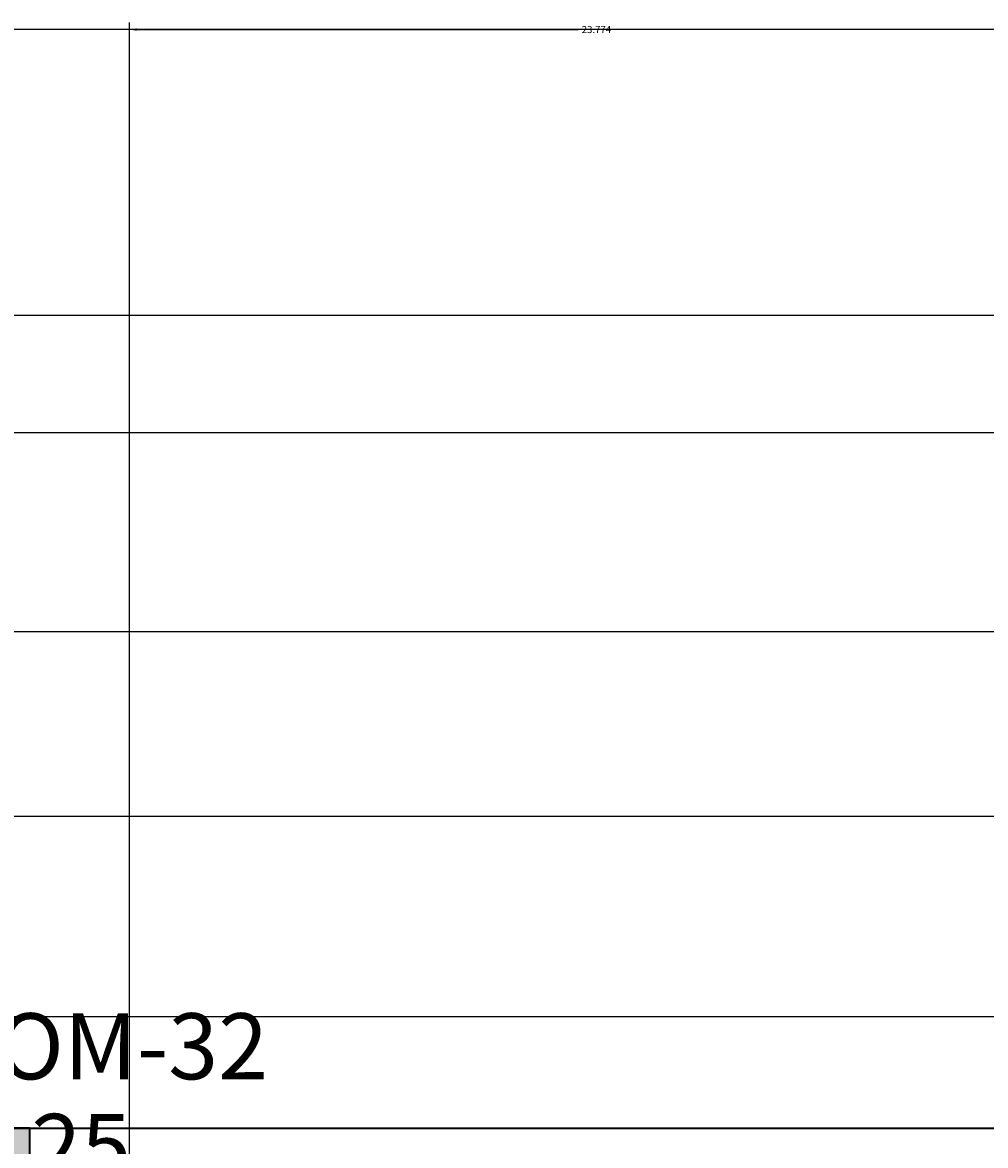
# Model space of a CAD drawing. Units: inches. Extents: x 23 to 132, y 5 to 105.
# Tile 13 of 14: x 81 to 105, y 77 to 105. Entities that reach past the tile are written whole.
import ezdxf

# ---------------------------------------------------------------- set-up
doc = ezdxf.new("R2010")
doc.units = ezdxf.units.IN
doc.header["$MEASUREMENT"] = 0
for name, color, linetype, lineweight in [('A-ANNO-DIMS', 2, 'Continuous', 18), ('E-ANNO-IDEN', 4, 'Continuous', 18), ('E-ANNO-TEXT', 3, 'Continuous', 18), ('E-SYMB', 1, 'Continuous', 35), ('E-SYMB-PATT', 1, 'Continuous', 18)]:
    doc.layers.add(name, color=color, linetype=linetype, lineweight=lineweight)
doc.styles.get("Standard").update_dxf_attribs({"font": 'arial.ttf'})
doc.dimstyles.get("Standard").update_dxf_attribs({"dimtxt": 0.18, "dimasz": 0.18, "dimexe": 0.18, "dimexo": 0.0625, "dimgap": 0.09, "dimtad": 0, "dimtih": 1, "dimtoh": 1, "dimdec": 4, "dimzin": 0, "dimdsep": 46, "dimtxsty": 'Standard', "dimcen": 0.09, "dimadec": 0, "dimazin": 0, "dimtfac": 1, "dimtdec": 4, "dimtofl": 0, "dimtmove": 0, "dimatfit": 3, "dimfxl": 1, "dimtolj": 1, "dimtzin": 0, "dimarcsym": 0})

# ---------------------------------------------------------------- blocks, each defined once
blk = doc.blocks.new('*D2')
at = {"layer": 'A-ANNO-DIMS', "color": 0, "lineweight": -2, "transparency": 16777216}
for p, q in [((28.697, 66.272), (28.697, 105.232)), ((123.211, 99.539), (123.211, 105.232)), ((28.877, 105.052), (75.577, 105.052)), ((123.031, 105.052), (76.33, 105.052))]:
    blk.add_line(p, q, dxfattribs=at)
at = {"layer": 'A-ANNO-DIMS', "color": 0, "transparency": 16777216}
for points in [[(28.877, 105.082), (28.877, 105.022), (28.697, 105.052)], [(123.031, 105.082), (123.031, 105.022), (123.211, 105.052)]]:
    blk.add_solid(points, dxfattribs=at)
at = {"layer": 'Defpoints', "color": 0, "transparency": 16777216}
for p in [(123.211, 105.052), (123.211, 99.477), (28.697, 66.21)]:
    blk.add_point(p, dxfattribs=at)
at = {"layer": 'A-ANNO-DIMS', "color": 0, "transparency": 16777216, "insert": (75.954, 105.052), "char_height": 0.18, "attachment_point": 5}
blk.add_mtext('\\A1;94.51', dxfattribs=at)
blk = doc.blocks.new('*D3')
at = {"layer": 'A-ANNO-DIMS', "color": 0, "lineweight": -2, "transparency": 16777216}
for p, q in [((121.409, 99.285), (129.239, 99.285)), ((129.059, 99.105), (129.059, 55.423)), ((129.059, 11.378), (129.059, 55.06)), ((72.981, 11.198), (129.239, 11.198))]:
    blk.add_line(p, q, dxfattribs=at)
at = {"layer": 'A-ANNO-DIMS', "color": 0, "transparency": 16777216}
for points in [[(129.029, 99.105), (129.089, 99.105), (129.059, 99.285)], [(129.029, 11.378), (129.089, 11.378), (129.059, 11.198)]]:
    blk.add_solid(points, dxfattribs=at)
at = {"layer": 'Defpoints', "color": 0, "transparency": 16777216}
for p in [(121.346, 99.285), (129.059, 99.285), (72.919, 11.198)]:
    blk.add_point(p, dxfattribs=at)
at = {"layer": 'A-ANNO-DIMS', "color": 0, "transparency": 16777216, "insert": (129.059, 55.241), "char_height": 0.18, "attachment_point": 5}
blk.add_mtext('\\A1;88.09', dxfattribs=at)
blk = doc.blocks.new('*D15')
at = {"layer": 'A-ANNO-DIMS', "color": 0, "lineweight": -2, "transparency": 16777216}
for p, q in [((50.327, 77.095), (129.239, 77.095)), ((129.059, 76.915), (129.059, 76.538)), ((129.059, 75.801), (129.059, 76.177)), ((47.783, 75.621), (129.239, 75.621))]:
    blk.add_line(p, q, dxfattribs=at)
at = {"layer": 'A-ANNO-DIMS', "color": 0, "transparency": 16777216}
for points in [[(129.029, 76.915), (129.089, 76.915), (129.059, 77.095)], [(129.029, 75.801), (129.089, 75.801), (129.059, 75.621)]]:
    blk.add_solid(points, dxfattribs=at)
at = {"layer": 'Defpoints', "color": 0, "transparency": 16777216}
for p in [(50.265, 77.095), (47.72, 75.621), (129.059, 75.621)]:
    blk.add_point(p, dxfattribs=at)
at = {"layer": 'A-ANNO-DIMS', "color": 0, "transparency": 16777216, "insert": (129.059, 76.358), "char_height": 0.18, "attachment_point": 5}
blk.add_mtext('\\A1;1.47', dxfattribs=at)
blk = doc.blocks.new('*D24')
at = {"layer": 'A-ANNO-DIMS', "color": 0, "lineweight": -2, "transparency": 16777216}
for p, q in [((81.032, 77.095), (129.239, 77.095)), ((129.059, 76.915), (129.059, 76.509)), ((129.059, 75.739), (129.059, 76.145)), ((83.576, 75.559), (129.239, 75.559))]:
    blk.add_line(p, q, dxfattribs=at)
at = {"layer": 'A-ANNO-DIMS', "color": 0, "transparency": 16777216}
for points in [[(129.029, 76.915), (129.089, 76.915), (129.059, 77.095)], [(129.029, 75.739), (129.089, 75.739), (129.059, 75.559)]]:
    blk.add_solid(points, dxfattribs=at)
at = {"layer": 'Defpoints', "color": 0, "transparency": 16777216}
for p in [(80.969, 77.095), (83.514, 75.559), (129.059, 75.559)]:
    blk.add_point(p, dxfattribs=at)
at = {"layer": 'A-ANNO-DIMS', "color": 0, "transparency": 16777216, "insert": (129.059, 76.327), "char_height": 0.18, "attachment_point": 5}
blk.add_mtext('\\A1;1.54', dxfattribs=at)
blk = doc.blocks.new('*D49')
at = {"layer": 'A-ANNO-DIMS', "color": 0, "lineweight": -2, "transparency": 16777216}
for p, q in [((83.514, 75.622), (83.514, 105.232)), ((107.287, 75.622), (107.287, 105.232)), ((83.694, 105.052), (94.936, 105.052)), ((107.107, 105.052), (95.865, 105.052))]:
    blk.add_line(p, q, dxfattribs=at)
at = {"layer": 'A-ANNO-DIMS', "color": 0, "transparency": 16777216}
for points in [[(83.694, 105.082), (83.694, 105.022), (83.514, 105.052)], [(107.107, 105.082), (107.107, 105.022), (107.287, 105.052)]]:
    blk.add_solid(points, dxfattribs=at)
at = {"layer": 'Defpoints', "color": 0, "transparency": 16777216}
for p in [(107.287, 105.052), (83.514, 75.559), (107.287, 75.559)]:
    blk.add_point(p, dxfattribs=at)
at = {"layer": 'A-ANNO-DIMS', "color": 0, "transparency": 16777216, "insert": (95.4, 105.052), "char_height": 0.18, "attachment_point": 5}
blk.add_mtext('\\A1;23.774', dxfattribs=at)
blk = doc.blocks.new('*D85')
at = {"layer": 'A-ANNO-DIMS', "color": 0, "lineweight": -2, "transparency": 16777216}
for p, q in [((106.903, 97.776), (22.942, 97.776)), ((23.122, 97.596), (23.122, 87.606)), ((23.122, 77.251), (23.122, 87.242)), ((106.964, 77.071), (22.942, 77.071))]:
    blk.add_line(p, q, dxfattribs=at)
at = {"layer": 'A-ANNO-DIMS', "color": 0, "transparency": 16777216}
for points in [[(23.092, 97.596), (23.152, 97.596), (23.122, 97.776)], [(23.092, 77.251), (23.152, 77.251), (23.122, 77.071)]]:
    blk.add_solid(points, dxfattribs=at)
at = {"layer": 'Defpoints', "color": 0, "transparency": 16777216}
for p in [(23.122, 97.776), (106.965, 97.776), (107.026, 77.071)]:
    blk.add_point(p, dxfattribs=at)
at = {"layer": 'A-ANNO-DIMS', "color": 0, "transparency": 16777216, "insert": (23.122, 87.424), "char_height": 0.18, "attachment_point": 5}
blk.add_mtext('\\A1;20.705', dxfattribs=at)
blk = doc.blocks.new('*D86')
at = {"layer": 'A-ANNO-DIMS', "color": 0, "lineweight": -2, "transparency": 16777216}
for p, q in [((110.027, 79.916), (22.942, 79.916)), ((23.122, 79.736), (23.122, 78.675)), ((23.122, 77.251), (23.122, 78.312)), ((106.964, 77.071), (22.942, 77.071))]:
    blk.add_line(p, q, dxfattribs=at)
at = {"layer": 'A-ANNO-DIMS', "color": 0, "transparency": 16777216}
for points in [[(23.092, 79.736), (23.152, 79.736), (23.122, 79.916)], [(23.092, 77.251), (23.152, 77.251), (23.122, 77.071)]]:
    blk.add_solid(points, dxfattribs=at)
at = {"layer": 'Defpoints', "color": 0, "transparency": 16777216}
for p in [(23.122, 79.916), (110.089, 79.916), (107.026, 77.071)]:
    blk.add_point(p, dxfattribs=at)
at = {"layer": 'A-ANNO-DIMS', "color": 0, "transparency": 16777216, "insert": (23.122, 78.493), "char_height": 0.18, "attachment_point": 5}
blk.add_mtext('\\A1;2.84', dxfattribs=at)
blk = doc.blocks.new('*D87')
at = {"layer": 'A-ANNO-DIMS', "color": 0, "lineweight": -2, "transparency": 16777216}
for p, q in [((110.027, 85.021), (22.942, 85.021)), ((23.122, 84.841), (23.122, 82.65)), ((23.122, 80.096), (23.122, 82.286)), ((110.027, 79.916), (22.942, 79.916))]:
    blk.add_line(p, q, dxfattribs=at)
at = {"layer": 'A-ANNO-DIMS', "color": 0, "transparency": 16777216}
for points in [[(23.092, 84.841), (23.152, 84.841), (23.122, 85.021)], [(23.092, 80.096), (23.152, 80.096), (23.122, 79.916)]]:
    blk.add_solid(points, dxfattribs=at)
at = {"layer": 'Defpoints', "color": 0, "transparency": 16777216}
for p in [(23.122, 85.021), (110.089, 85.021), (110.089, 79.916)]:
    blk.add_point(p, dxfattribs=at)
at = {"layer": 'A-ANNO-DIMS', "color": 0, "transparency": 16777216, "insert": (23.122, 82.468), "char_height": 0.18, "attachment_point": 5}
blk.add_mtext('\\A1;5.105', dxfattribs=at)
blk = doc.blocks.new('*D88')
at = {"layer": 'A-ANNO-DIMS', "color": 0, "lineweight": -2, "transparency": 16777216}
for p, q in [((110.027, 89.722), (22.942, 89.722)), ((23.122, 89.542), (23.122, 87.554)), ((23.122, 85.201), (23.122, 87.19)), ((110.027, 85.021), (22.942, 85.021))]:
    blk.add_line(p, q, dxfattribs=at)
at = {"layer": 'A-ANNO-DIMS', "color": 0, "transparency": 16777216}
for points in [[(23.092, 89.542), (23.152, 89.542), (23.122, 89.722)], [(23.092, 85.201), (23.152, 85.201), (23.122, 85.021)]]:
    blk.add_solid(points, dxfattribs=at)
at = {"layer": 'Defpoints', "color": 0, "transparency": 16777216}
for p in [(23.122, 89.722), (110.089, 89.722), (110.089, 85.021)]:
    blk.add_point(p, dxfattribs=at)
at = {"layer": 'A-ANNO-DIMS', "color": 0, "transparency": 16777216, "insert": (23.122, 87.372), "char_height": 0.18, "attachment_point": 5}
blk.add_mtext('\\A1;4.702', dxfattribs=at)
blk = doc.blocks.new('*D89')
at = {"layer": 'A-ANNO-DIMS', "color": 0, "lineweight": -2, "transparency": 16777216}
for p, q in [((110.298, 94.783), (22.942, 94.783)), ((23.122, 94.603), (23.122, 92.435)), ((23.122, 89.902), (23.122, 92.071)), ((110.027, 89.722), (22.942, 89.722))]:
    blk.add_line(p, q, dxfattribs=at)
at = {"layer": 'A-ANNO-DIMS', "color": 0, "transparency": 16777216}
for points in [[(23.092, 94.603), (23.152, 94.603), (23.122, 94.783)], [(23.092, 89.902), (23.152, 89.902), (23.122, 89.722)]]:
    blk.add_solid(points, dxfattribs=at)
at = {"layer": 'Defpoints', "color": 0, "transparency": 16777216}
for p in [(23.122, 94.783), (110.36, 94.783), (110.089, 89.722)]:
    blk.add_point(p, dxfattribs=at)
at = {"layer": 'A-ANNO-DIMS', "color": 0, "transparency": 16777216, "insert": (23.122, 92.253), "char_height": 0.18, "attachment_point": 5}
blk.add_mtext('\\A1;5.061', dxfattribs=at)
blk = doc.blocks.new('*D90')
at = {"layer": 'A-ANNO-DIMS', "color": 0, "lineweight": -2, "transparency": 16777216}
for p, q in [((106.903, 97.776), (22.942, 97.776)), ((23.122, 97.596), (23.122, 96.462)), ((23.122, 94.963), (23.122, 96.098)), ((110.298, 94.783), (22.942, 94.783))]:
    blk.add_line(p, q, dxfattribs=at)
at = {"layer": 'A-ANNO-DIMS', "color": 0, "transparency": 16777216}
for points in [[(23.092, 97.596), (23.152, 97.596), (23.122, 97.776)], [(23.092, 94.963), (23.152, 94.963), (23.122, 94.783)]]:
    blk.add_solid(points, dxfattribs=at)
at = {"layer": 'Defpoints', "color": 0, "transparency": 16777216}
for p in [(23.122, 97.776), (106.965, 97.776), (110.36, 94.783)]:
    blk.add_point(p, dxfattribs=at)
at = {"layer": 'A-ANNO-DIMS', "color": 0, "transparency": 16777216, "insert": (23.122, 96.28), "char_height": 0.18, "attachment_point": 5}
blk.add_mtext('\\A1;2.993', dxfattribs=at)

msp = doc.modelspace()

# ---------------------------------------------------------------- hatches: boundary and pattern name
at = {"layer": 'E-SYMB-PATT'}
h = msp.add_hatch(color=256, dxfattribs=at)
h.dxf.hatch_style = 1
h.paths.add_polyline_path([(80.9692, 77.095), (50.2646, 77.095), (50.2646, 18.0066), (80.9692, 18.0066)])

# ---------------------------------------------------------------- linework, layer by layer
at = {"layer": 'E-SYMB'}
msp.add_lwpolyline([(50.2646, 77.095), (80.9692, 77.095), (80.9692, 18.0066), (50.2646, 18.0066)], close=True, dxfattribs=at)

# ---------------------------------------------------------------- texts
at = {"layer": 'E-ANNO-IDEN'}
msp.add_text('ESP32-WROOM-32', height=1.679435, dxfattribs=at).set_placement((67.4727, 78.3292))
at = {"layer": 'E-ANNO-TEXT'}
msp.add_text('25', height=1.67943, dxfattribs=at).set_placement((81.0136, 75.7678))

# ---------------------------------------------------------------- dimensions: what is measured, and where the dimension line sits
at = {"layer": 'A-ANNO-DIMS'}
for base, p1, p2, override, picture, middle in [((123.2107, 105.052), (28.6965, 66.2099), (123.2107, 99.477), {"dimdec": 2, "dimlfac": 1, "dimrnd": 0, "dimzin": 0, "dimdsep": 46, "dimlunit": 2}, '*D2', (75.9536, 105.052)), ((107.2874, 105.052), (83.5136, 75.5594), (107.2874, 75.5594), {"dimdec": 3, "dimlfac": 1, "dimrnd": 0, "dimzin": 0, "dimdsep": 46, "dimlunit": 2}, '*D49', (95.4005, 105.052))]:
    dim = msp.add_linear_dim(base=base, p1=p1, p2=p2, dimstyle='Standard', override=override, dxfattribs=at)
    dim.commit()
    dim.dimension.update_dxf_attribs({"geometry": picture, "text_midpoint": middle})
for base, p1, p2, override, picture, middle in [((129.0589, 99.2846), (72.9188, 11.1983), (121.3461, 99.2846), {"dimdec": 2, "dimlfac": 1, "dimrnd": 0, "dimzin": 0, "dimdsep": 46, "dimlunit": 2}, '*D3', (129.0589, 55.2415)), ((23.1215, 97.7764), (107.026, 77.0711), (106.9652, 97.7764), {"dimdec": 3, "dimlfac": 1, "dimrnd": 0, "dimzin": 0, "dimdsep": 46, "dimlunit": 2}, '*D85', (23.1215, 87.4238)), ((23.1215, 97.7764), (110.36, 94.7833), (106.9652, 97.7764), {"dimdec": 3, "dimlfac": 1, "dimrnd": 0, "dimzin": 0, "dimdsep": 46, "dimlunit": 2}, '*D90', (23.1215, 96.2798)), ((23.1215, 94.7833), (110.0892, 89.7224), (110.36, 94.7833), {"dimdec": 3, "dimlfac": 1, "dimrnd": 0, "dimzin": 0, "dimdsep": 46, "dimlunit": 2}, '*D89', (23.1215, 92.2528)), ((23.12152, 89.7224), (110.08916, 85.02085), (110.08916, 89.7224), {"dimdec": 3, "dimlfac": 1, "dimrnd": 0, "dimzin": 0, "dimdsep": 46, "dimlunit": 2}, '*D88', (23.12152, 87.37162)), ((23.1215, 85.0209), (110.0892, 79.9158), (110.0892, 85.0209), {"dimdec": 3, "dimlfac": 1, "dimrnd": 0, "dimzin": 0, "dimdsep": 46, "dimlunit": 2}, '*D87', (23.1215, 82.4683)), ((23.1215, 79.9158), (107.026, 77.0711), (110.0892, 79.9158), {"dimdec": 2, "dimlfac": 1, "dimrnd": 0, "dimzin": 0, "dimdsep": 46, "dimlunit": 2}, '*D86', (23.1215, 78.4935)), ((129.0589, 75.6207), (50.2646, 77.095), (47.7202, 75.6207), {"dimdec": 2, "dimlfac": 1, "dimrnd": 0, "dimzin": 0, "dimdsep": 46, "dimlunit": 2}, '*D15', (129.0589, 76.3579)), ((129.0589, 75.5594), (80.9692, 77.095), (83.5136, 75.5594), {"dimdec": 2, "dimlfac": 1, "dimrnd": 0, "dimzin": 0, "dimdsep": 46, "dimlunit": 2}, '*D24', (129.0589, 76.3272))]:
    dim = msp.add_linear_dim(base=base, p1=p1, p2=p2, angle=90, dimstyle='Standard', override=override, dxfattribs=at)
    dim.commit()
    dim.dimension.update_dxf_attribs({"geometry": picture, "text_midpoint": middle})

doc.saveas('drawing.dxf')
